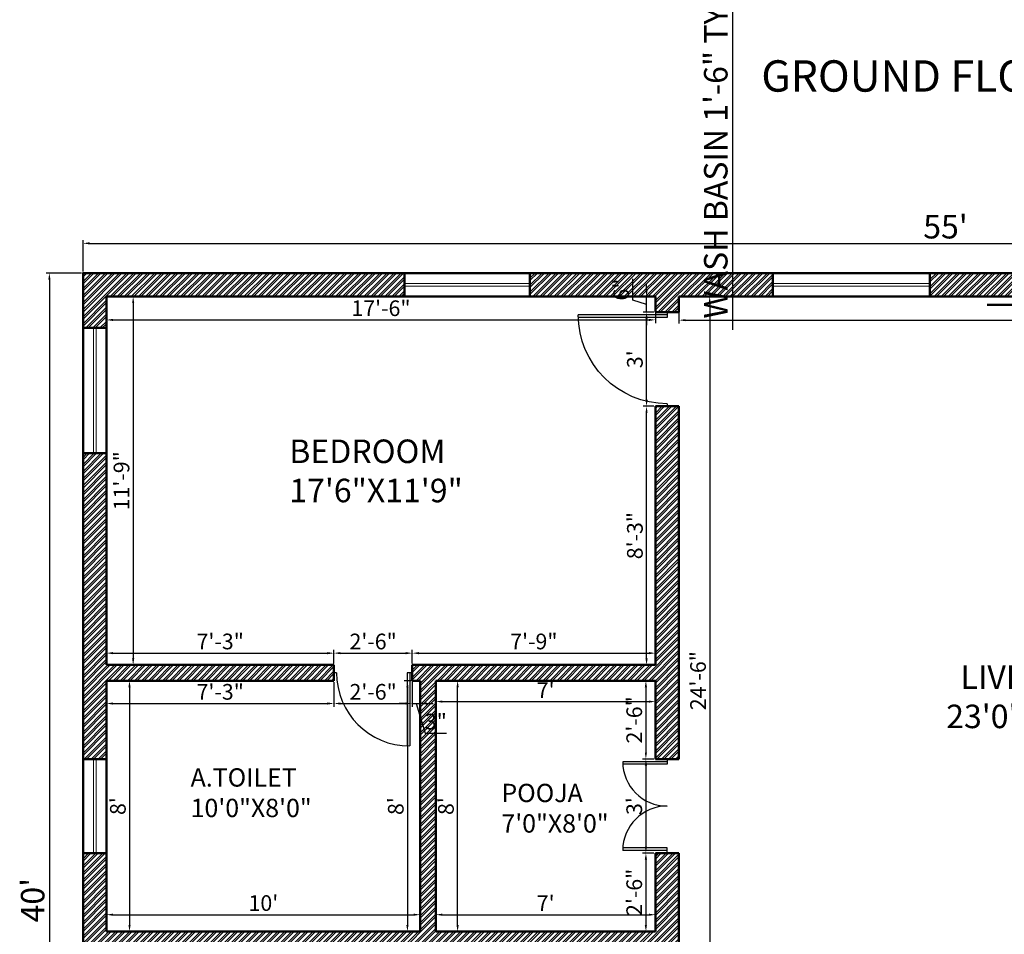
# Model space of a CAD drawing. Units: inches. Extents: x 3590 to 5167, y 65 to 1917.
# Tile 14 of 100: x 3621 to 3998, y 962 to 1312. Entities that reach past the tile are written whole.
import ezdxf

# ---------------------------------------------------------------- set-up
doc = ezdxf.new("R2010")
doc.units = ezdxf.units.IN
for name, color, linetype, lineweight in [('A-ANNO-DIMS', 2, 'Continuous', 18), ('A-ANNO-TEXT', 7, 'Continuous', 25), ('A-AREA-IDEN', 7, 'Continuous', 18), ('A-DOOR', 3, 'Continuous', 25), ('A-GLAZ', 4, 'Continuous', 18), ('A-WALL', 7, 'Continuous', 50), ('A-WALL-PATT', 251, 'Continuous', 13)]:
    doc.layers.add(name, color=color, linetype=linetype, lineweight=lineweight)
doc.styles.get("Standard").update_dxf_attribs({"font": 'arial.ttf'})
doc.dimstyles.new('ISO-25', dxfattribs={"dimtxt": 9, "dimasz": 2.5, "dimexe": 1.25, "dimexo": 0.625, "dimtad": 1, "dimdec": 1, "dimlunit": 3, "dimtxsty": 'Standard', "dimcen": 2.5, "dimadec": 0, "dimazin": 0, "dimtfac": 1, "dimtdec": 1, "dimtmove": 0, "dimatfit": 3, "dimfxl": 1, "dimarcsym": 0})

# ---------------------------------------------------------------- blocks, each defined once
blk = doc.blocks.new('*D9')
at = {"layer": 'A-ANNO-DIMS', "color": 0, "lineweight": -2, "transparency": 16777216}
for p, q in [((3645.51, 1215.97), (3645.51, 1227.96)), ((3648.01, 1226.71), (4303.01, 1226.71)), ((4305.51, 1215.97), (4305.51, 1227.96))]:
    blk.add_line(p, q, dxfattribs=at)
at = {"layer": 'A-ANNO-DIMS', "color": 0, "transparency": 16777216}
for points in [[(3648.01, 1227.13), (3648.01, 1226.29), (3645.51, 1226.71)], [(4303.01, 1227.13), (4303.01, 1226.29), (4305.51, 1226.71)]]:
    blk.add_solid(points, dxfattribs=at)
at = {"layer": 'Defpoints', "color": 0, "transparency": 16777216}
for p in [(4305.51, 1226.71), (3645.51, 1215.35), (4305.51, 1215.35)]:
    blk.add_point(p, dxfattribs=at)
at = {"layer": 'A-ANNO-DIMS', "color": 0, "transparency": 16777216, "insert": (3975.51, 1231.91), "char_height": 9, "attachment_point": 5}
blk.add_mtext("55'", dxfattribs=at)
blk = doc.blocks.new('*D10')
at = {"layer": 'A-ANNO-DIMS', "color": 0, "lineweight": -2, "transparency": 16777216}
for p, q in [((3644.89, 1215.35), (3631.39, 1215.35)), ((3632.64, 1212.85), (3632.64, 737.85)), ((3644.89, 735.35), (3631.39, 735.35))]:
    blk.add_line(p, q, dxfattribs=at)
at = {"layer": 'A-ANNO-DIMS', "color": 0, "transparency": 16777216}
for points in [[(3632.22, 1212.85), (3633.06, 1212.85), (3632.64, 1215.35)], [(3632.22, 737.85), (3633.06, 737.85), (3632.64, 735.35)]]:
    blk.add_solid(points, dxfattribs=at)
at = {"layer": 'Defpoints', "color": 0, "transparency": 16777216}
for p in [(3645.51, 1215.35), (3632.64, 735.35), (3645.51, 735.35)]:
    blk.add_point(p, dxfattribs=at)
at = {"layer": 'A-ANNO-DIMS', "color": 0, "transparency": 16777216, "insert": (3627.42, 975.35), "char_height": 9, "attachment_point": 5, "rotation": 90}
blk.add_mtext("40'", dxfattribs=at)
blk = doc.blocks.new('D1')
for p, q in [((1, 0), (1, 34)), ((2, 0), (2, 33.99)), ((0, 0), (2, 0)), ((35, 0), (36, 0))]:
    blk.add_line(p, q)
at = {"ltscale": 0.5}
blk.add_arc((1, 0), 34, 0, 90, dxfattribs=at)
blk = doc.blocks.new('D2')
for p, q in [((1, 0), (1, 28)), ((2, 0), (2, 27.98)), ((0, 0), (2, 0)), ((29, 0), (30, 0))]:
    blk.add_line(p, q)
at = {"ltscale": 0.5}
blk.add_arc((1, 0), 28, 0, 90, dxfattribs=at)
blk = doc.blocks.new('D3')
for p, q in [((1, 0), (1, 17)), ((2, 0), (2, 16.97)), ((34, 0), (34, 16.97)), ((35, 0), (35, 17)), ((0, 0), (2, 0)), ((36, 0), (34, 0))]:
    blk.add_line(p, q)
at = {"ltscale": 0.5}
for centre, start, end in [((1, 0), 0, 90), ((35, 0), 90, 180)]:
    blk.add_arc(centre, 17, start, end, dxfattribs=at)
blk = doc.blocks.new('*D15')
at = {"layer": 'A-ANNO-DIMS', "color": 0, "lineweight": -2, "transparency": 16777216}
for p, q in [((3654.51, 1205.72), (3654.51, 1196.16)), ((3864.51, 1205.72), (3864.51, 1196.16)), ((3657.01, 1197.41), (3862.01, 1197.41))]:
    blk.add_line(p, q, dxfattribs=at)
at = {"layer": 'A-ANNO-DIMS', "color": 0, "transparency": 16777216}
for points in [[(3657.01, 1197.82), (3657.01, 1196.99), (3654.51, 1197.41)], [(3862.01, 1197.82), (3862.01, 1196.99), (3864.51, 1197.41)]]:
    blk.add_solid(points, dxfattribs=at)
at = {"layer": 'Defpoints', "color": 0, "transparency": 16777216}
for p in [(3654.51, 1206.35), (3864.51, 1206.35), (3864.51, 1197.41)]:
    blk.add_point(p, dxfattribs=at)
at = {"layer": 'A-ANNO-DIMS', "color": 0, "transparency": 16777216, "insert": (3759.51, 1201.1), "char_height": 6, "attachment_point": 5}
blk.add_mtext('17\'-6"', dxfattribs=at)
blk = doc.blocks.new('*D16')
at = {"layer": 'A-ANNO-DIMS', "color": 0, "lineweight": -2, "transparency": 16777216}
for p, q in [((3655.14, 1206.35), (3665.95, 1206.35)), ((3664.7, 1203.85), (3664.7, 1067.85)), ((3655.14, 1065.35), (3665.95, 1065.35))]:
    blk.add_line(p, q, dxfattribs=at)
at = {"layer": 'A-ANNO-DIMS', "color": 0, "transparency": 16777216}
for points in [[(3664.29, 1203.85), (3665.12, 1203.85), (3664.7, 1206.35)], [(3664.29, 1067.85), (3665.12, 1067.85), (3664.7, 1065.35)]]:
    blk.add_solid(points, dxfattribs=at)
at = {"layer": 'Defpoints', "color": 0, "transparency": 16777216}
for p in [(3654.51, 1206.35), (3654.51, 1065.35), (3664.7, 1065.35)]:
    blk.add_point(p, dxfattribs=at)
at = {"layer": 'A-ANNO-DIMS', "color": 0, "transparency": 16777216, "insert": (3661.02, 1135.85), "char_height": 6, "attachment_point": 5, "rotation": 90}
blk.add_mtext('11\'-9"', dxfattribs=at)
blk = doc.blocks.new('*D17')
at = {"layer": 'A-ANNO-DIMS', "color": 0, "lineweight": -2, "transparency": 16777216}
for p, q in [((3654.51, 1065.97), (3654.51, 1071.13)), ((3741.51, 1065.97), (3741.51, 1071.13)), ((3657.01, 1069.88), (3739.01, 1069.88))]:
    blk.add_line(p, q, dxfattribs=at)
at = {"layer": 'A-ANNO-DIMS', "color": 0, "transparency": 16777216}
for points in [[(3657.01, 1070.3), (3657.01, 1069.46), (3654.51, 1069.88)], [(3739.01, 1070.3), (3739.01, 1069.46), (3741.51, 1069.88)]]:
    blk.add_solid(points, dxfattribs=at)
at = {"layer": 'Defpoints', "color": 0, "transparency": 16777216}
for p in [(3741.51, 1069.88), (3654.51, 1065.35), (3741.51, 1065.35)]:
    blk.add_point(p, dxfattribs=at)
at = {"layer": 'A-ANNO-DIMS', "color": 0, "transparency": 16777216, "insert": (3698.01, 1073.57), "char_height": 6, "attachment_point": 5}
blk.add_mtext('7\'-3"', dxfattribs=at)
blk = doc.blocks.new('*D18')
at = {"layer": 'A-ANNO-DIMS', "color": 0, "lineweight": -2, "transparency": 16777216}
for p, q in [((3741.51, 1065.97), (3741.51, 1071.13)), ((3771.51, 1065.97), (3771.51, 1071.13)), ((3744.01, 1069.88), (3769.01, 1069.88))]:
    blk.add_line(p, q, dxfattribs=at)
at = {"layer": 'A-ANNO-DIMS', "color": 0, "transparency": 16777216}
for points in [[(3744.01, 1070.3), (3744.01, 1069.46), (3741.51, 1069.88)], [(3769.01, 1070.3), (3769.01, 1069.46), (3771.51, 1069.88)]]:
    blk.add_solid(points, dxfattribs=at)
at = {"layer": 'Defpoints', "color": 0, "transparency": 16777216}
for p in [(3771.51, 1069.88), (3741.51, 1065.35), (3771.51, 1065.35)]:
    blk.add_point(p, dxfattribs=at)
at = {"layer": 'A-ANNO-DIMS', "color": 0, "transparency": 16777216, "insert": (3756.51, 1073.57), "char_height": 6, "attachment_point": 5}
blk.add_mtext('2\'-6"', dxfattribs=at)
blk = doc.blocks.new('*D19')
at = {"layer": 'A-ANNO-DIMS', "color": 0, "lineweight": -2, "transparency": 16777216}
for p, q in [((3771.51, 1065.97), (3771.51, 1071.13)), ((3864.51, 1065.97), (3864.51, 1071.13)), ((3774.01, 1069.88), (3862.01, 1069.88))]:
    blk.add_line(p, q, dxfattribs=at)
at = {"layer": 'A-ANNO-DIMS', "color": 0, "transparency": 16777216}
for points in [[(3774.01, 1070.3), (3774.01, 1069.46), (3771.51, 1069.88)], [(3862.01, 1070.3), (3862.01, 1069.46), (3864.51, 1069.88)]]:
    blk.add_solid(points, dxfattribs=at)
at = {"layer": 'Defpoints', "color": 0, "transparency": 16777216}
for p in [(3864.51, 1069.88), (3771.51, 1065.35), (3864.51, 1065.35)]:
    blk.add_point(p, dxfattribs=at)
at = {"layer": 'A-ANNO-DIMS', "color": 0, "transparency": 16777216, "insert": (3818.01, 1073.57), "char_height": 6, "attachment_point": 5}
blk.add_mtext('7\'-9"', dxfattribs=at)
blk = doc.blocks.new('*D20')
at = {"layer": 'A-ANNO-DIMS', "color": 0, "lineweight": -2, "transparency": 16777216}
for p, q in [((3863.89, 1164.35), (3859.88, 1164.35)), ((3861.13, 1067.85), (3861.13, 1161.85)), ((3863.89, 1065.35), (3859.88, 1065.35))]:
    blk.add_line(p, q, dxfattribs=at)
at = {"layer": 'A-ANNO-DIMS', "color": 0, "transparency": 16777216}
for points in [[(3860.71, 1161.85), (3861.55, 1161.85), (3861.13, 1164.35)], [(3860.71, 1067.85), (3861.55, 1067.85), (3861.13, 1065.35)]]:
    blk.add_solid(points, dxfattribs=at)
at = {"layer": 'Defpoints', "color": 0, "transparency": 16777216}
for p in [(3861.13, 1164.35), (3864.51, 1164.35), (3864.51, 1065.35)]:
    blk.add_point(p, dxfattribs=at)
at = {"layer": 'A-ANNO-DIMS', "color": 0, "transparency": 16777216, "insert": (3857.44, 1114.85), "char_height": 6, "attachment_point": 5, "rotation": 90}
blk.add_mtext('8\'-3"', dxfattribs=at)
blk = doc.blocks.new('*D21')
at = {"layer": 'A-ANNO-DIMS', "color": 0, "lineweight": -2, "transparency": 16777216}
for p, q in [((3863.89, 1200.35), (3859.88, 1200.35)), ((3861.13, 1166.85), (3861.13, 1197.85)), ((3863.89, 1164.35), (3859.88, 1164.35))]:
    blk.add_line(p, q, dxfattribs=at)
at = {"layer": 'A-ANNO-DIMS', "color": 0, "transparency": 16777216}
for points in [[(3860.71, 1197.85), (3861.55, 1197.85), (3861.13, 1200.35)], [(3860.71, 1166.85), (3861.55, 1166.85), (3861.13, 1164.35)]]:
    blk.add_solid(points, dxfattribs=at)
at = {"layer": 'Defpoints', "color": 0, "transparency": 16777216}
for p in [(3861.13, 1200.35), (3864.51, 1200.35), (3864.51, 1164.35)]:
    blk.add_point(p, dxfattribs=at)
at = {"layer": 'A-ANNO-DIMS', "color": 0, "transparency": 16777216, "insert": (3857.44, 1182.35), "char_height": 6, "attachment_point": 5, "rotation": 90}
blk.add_mtext("3'", dxfattribs=at)
blk = doc.blocks.new('*D22')
at = {"layer": 'A-ANNO-DIMS', "color": 0, "lineweight": -2, "transparency": 16777216}
for p, q in [((3855.88, 1204.92), (3855.88, 1213.1)), ((3861.13, 1208.85), (3861.13, 1211.35)), ((3863.89, 1206.35), (3859.88, 1206.35)), ((3861.13, 1200.35), (3861.13, 1206.35)), ((3861.13, 1200.35), (3861.13, 1206.35)), ((3861.13, 1203.35), (3855.88, 1204.92)), ((3863.89, 1200.35), (3859.88, 1200.35)), ((3861.13, 1197.85), (3861.13, 1195.35))]:
    blk.add_line(p, q, dxfattribs=at)
at = {"layer": 'A-ANNO-DIMS', "color": 0, "transparency": 16777216}
for points in [[(3860.71, 1208.85), (3861.55, 1208.85), (3861.13, 1206.35)], [(3860.71, 1197.85), (3861.55, 1197.85), (3861.13, 1200.35)]]:
    blk.add_solid(points, dxfattribs=at)
at = {"layer": 'Defpoints', "color": 0, "transparency": 16777216}
for p in [(3861.13, 1206.35), (3864.51, 1206.35), (3864.51, 1200.35)]:
    blk.add_point(p, dxfattribs=at)
at = {"layer": 'A-ANNO-DIMS', "color": 0, "transparency": 16777216, "insert": (3852.19, 1209.01), "char_height": 6, "attachment_point": 5, "rotation": 90}
blk.add_mtext('6"', dxfattribs=at)
blk = doc.blocks.new('*D23')
at = {"layer": 'A-ANNO-DIMS', "color": 0, "lineweight": -2, "transparency": 16777216}
for p, q in [((3654.51, 1058.72), (3654.51, 1049.36)), ((3741.51, 1058.72), (3741.51, 1049.36)), ((3657.01, 1050.61), (3739.01, 1050.61))]:
    blk.add_line(p, q, dxfattribs=at)
at = {"layer": 'A-ANNO-DIMS', "color": 0, "transparency": 16777216}
for points in [[(3657.01, 1051.03), (3657.01, 1050.19), (3654.51, 1050.61)], [(3739.01, 1051.03), (3739.01, 1050.19), (3741.51, 1050.61)]]:
    blk.add_solid(points, dxfattribs=at)
at = {"layer": 'Defpoints', "color": 0, "transparency": 16777216}
for p in [(3654.51, 1059.35), (3741.51, 1059.35), (3741.51, 1050.61)]:
    blk.add_point(p, dxfattribs=at)
at = {"layer": 'A-ANNO-DIMS', "color": 0, "transparency": 16777216, "insert": (3698.01, 1054.3), "char_height": 6, "attachment_point": 5}
blk.add_mtext('7\'-3"', dxfattribs=at)
blk = doc.blocks.new('*D24')
at = {"layer": 'A-ANNO-DIMS', "color": 0, "lineweight": -2, "transparency": 16777216}
for p, q in [((3741.51, 1058.72), (3741.51, 1049.36)), ((3771.51, 1058.72), (3771.51, 1049.36)), ((3744.01, 1050.61), (3769.01, 1050.61))]:
    blk.add_line(p, q, dxfattribs=at)
at = {"layer": 'A-ANNO-DIMS', "color": 0, "transparency": 16777216}
for points in [[(3744.01, 1051.03), (3744.01, 1050.19), (3741.51, 1050.61)], [(3769.01, 1051.03), (3769.01, 1050.19), (3771.51, 1050.61)]]:
    blk.add_solid(points, dxfattribs=at)
at = {"layer": 'Defpoints', "color": 0, "transparency": 16777216}
for p in [(3741.51, 1059.35), (3771.51, 1059.35), (3771.51, 1050.61)]:
    blk.add_point(p, dxfattribs=at)
at = {"layer": 'A-ANNO-DIMS', "color": 0, "transparency": 16777216, "insert": (3756.51, 1054.3), "char_height": 6, "attachment_point": 5}
blk.add_mtext('2\'-6"', dxfattribs=at)
blk = doc.blocks.new('*D25')
at = {"layer": 'A-ANNO-DIMS', "color": 0, "lineweight": -2, "transparency": 16777216}
for p, q in [((3771.51, 1058.72), (3771.51, 1049.36)), ((3774.51, 1058.72), (3774.51, 1049.36)), ((3769.01, 1050.61), (3766.51, 1050.61)), ((3771.51, 1050.61), (3774.51, 1050.61)), ((3771.51, 1050.61), (3774.51, 1050.61)), ((3773.01, 1050.61), (3776.43, 1039.23)), ((3777.01, 1050.61), (3779.51, 1050.61)), ((3776.43, 1039.23), (3784.57, 1039.23))]:
    blk.add_line(p, q, dxfattribs=at)
at = {"layer": 'A-ANNO-DIMS', "color": 0, "transparency": 16777216}
for points in [[(3769.01, 1051.03), (3769.01, 1050.19), (3771.51, 1050.61)], [(3777.01, 1051.03), (3777.01, 1050.19), (3774.51, 1050.61)]]:
    blk.add_solid(points, dxfattribs=at)
at = {"layer": 'Defpoints', "color": 0, "transparency": 16777216}
for p in [(3771.51, 1059.35), (3774.51, 1059.35), (3774.51, 1050.61)]:
    blk.add_point(p, dxfattribs=at)
at = {"layer": 'A-ANNO-DIMS', "color": 0, "transparency": 16777216, "insert": (3780.5, 1042.92), "char_height": 6, "attachment_point": 5}
blk.add_mtext('3"', dxfattribs=at)
blk = doc.blocks.new('*D26')
at = {"layer": 'A-ANNO-DIMS', "color": 0, "lineweight": -2, "transparency": 16777216}
for p, q in [((3655.14, 1059.35), (3664.56, 1059.35)), ((3663.31, 1056.85), (3663.31, 965.85)), ((3655.14, 963.35), (3664.56, 963.35))]:
    blk.add_line(p, q, dxfattribs=at)
at = {"layer": 'A-ANNO-DIMS', "color": 0, "transparency": 16777216}
for points in [[(3662.89, 1056.85), (3663.72, 1056.85), (3663.31, 1059.35)], [(3662.89, 965.85), (3663.72, 965.85), (3663.31, 963.35)]]:
    blk.add_solid(points, dxfattribs=at)
at = {"layer": 'Defpoints', "color": 0, "transparency": 16777216}
for p in [(3654.51, 1059.35), (3654.51, 963.35), (3663.31, 963.35)]:
    blk.add_point(p, dxfattribs=at)
at = {"layer": 'A-ANNO-DIMS', "color": 0, "transparency": 16777216, "insert": (3659.62, 1011.35), "char_height": 6, "attachment_point": 5, "rotation": 90}
blk.add_mtext("8'", dxfattribs=at)
blk = doc.blocks.new('*D27')
at = {"layer": 'A-ANNO-DIMS', "color": 0, "lineweight": -2, "transparency": 16777216}
for p, q in [((3654.51, 963.97), (3654.51, 971.04)), ((3657.01, 969.79), (3772.01, 969.79)), ((3774.51, 963.97), (3774.51, 971.04))]:
    blk.add_line(p, q, dxfattribs=at)
at = {"layer": 'A-ANNO-DIMS', "color": 0, "transparency": 16777216}
for points in [[(3657.01, 970.2), (3657.01, 969.37), (3654.51, 969.79)], [(3772.01, 970.2), (3772.01, 969.37), (3774.51, 969.79)]]:
    blk.add_solid(points, dxfattribs=at)
at = {"layer": 'Defpoints', "color": 0, "transparency": 16777216}
for p in [(3774.51, 969.79), (3654.51, 963.35), (3774.51, 963.35)]:
    blk.add_point(p, dxfattribs=at)
at = {"layer": 'A-ANNO-DIMS', "color": 0, "transparency": 16777216, "insert": (3714.51, 973.47), "char_height": 6, "attachment_point": 5}
blk.add_mtext("10'", dxfattribs=at)
blk = doc.blocks.new('*D28')
at = {"layer": 'A-ANNO-DIMS', "color": 0, "lineweight": -2, "transparency": 16777216}
for p, q in [((3780.51, 963.97), (3780.51, 971.04)), ((3783.01, 969.79), (3862.01, 969.79)), ((3864.51, 963.97), (3864.51, 971.04))]:
    blk.add_line(p, q, dxfattribs=at)
at = {"layer": 'A-ANNO-DIMS', "color": 0, "transparency": 16777216}
for points in [[(3783.01, 970.2), (3783.01, 969.37), (3780.51, 969.79)], [(3862.01, 970.2), (3862.01, 969.37), (3864.51, 969.79)]]:
    blk.add_solid(points, dxfattribs=at)
at = {"layer": 'Defpoints', "color": 0, "transparency": 16777216}
for p in [(3864.51, 969.79), (3780.51, 963.35), (3864.51, 963.35)]:
    blk.add_point(p, dxfattribs=at)
at = {"layer": 'A-ANNO-DIMS', "color": 0, "transparency": 16777216, "insert": (3822.51, 973.41), "char_height": 6, "attachment_point": 5}
blk.add_mtext("7'", dxfattribs=at)
blk = doc.blocks.new('*D29')
at = {"layer": 'A-ANNO-DIMS', "color": 0, "lineweight": -2, "transparency": 16777216}
for p, q in [((3781.14, 1059.35), (3790.09, 1059.35)), ((3788.84, 965.85), (3788.84, 1056.85)), ((3781.14, 963.35), (3790.09, 963.35))]:
    blk.add_line(p, q, dxfattribs=at)
at = {"layer": 'A-ANNO-DIMS', "color": 0, "transparency": 16777216}
for points in [[(3788.42, 1056.85), (3789.26, 1056.85), (3788.84, 1059.35)], [(3788.42, 965.85), (3789.26, 965.85), (3788.84, 963.35)]]:
    blk.add_solid(points, dxfattribs=at)
at = {"layer": 'Defpoints', "color": 0, "transparency": 16777216}
for p in [(3780.51, 1059.35), (3788.84, 1059.35), (3780.51, 963.35)]:
    blk.add_point(p, dxfattribs=at)
at = {"layer": 'A-ANNO-DIMS', "color": 0, "transparency": 16777216, "insert": (3785.15, 1011.35), "char_height": 6, "attachment_point": 5, "rotation": 90}
blk.add_mtext("8'", dxfattribs=at)
blk = doc.blocks.new('*D30')
at = {"layer": 'A-ANNO-DIMS', "color": 0, "lineweight": -2, "transparency": 16777216}
for p, q in [((3773.89, 1059.35), (3768.39, 1059.35)), ((3769.64, 1056.85), (3769.64, 965.85)), ((3773.89, 963.35), (3768.39, 963.35))]:
    blk.add_line(p, q, dxfattribs=at)
at = {"layer": 'A-ANNO-DIMS', "color": 0, "transparency": 16777216}
for points in [[(3769.23, 1056.85), (3770.06, 1056.85), (3769.64, 1059.35)], [(3769.23, 965.85), (3770.06, 965.85), (3769.64, 963.35)]]:
    blk.add_solid(points, dxfattribs=at)
at = {"layer": 'Defpoints', "color": 0, "transparency": 16777216}
for p in [(3774.51, 1059.35), (3769.64, 963.35), (3774.51, 963.35)]:
    blk.add_point(p, dxfattribs=at)
at = {"layer": 'A-ANNO-DIMS', "color": 0, "transparency": 16777216, "insert": (3765.96, 1011.35), "char_height": 6, "attachment_point": 5, "rotation": 90}
blk.add_mtext("8'", dxfattribs=at)
blk = doc.blocks.new('*D31')
at = {"layer": 'A-ANNO-DIMS', "color": 0, "lineweight": -2, "transparency": 16777216}
for p, q in [((3780.51, 1058.72), (3780.51, 1050.09)), ((3864.51, 1058.72), (3864.51, 1050.09)), ((3783.01, 1051.34), (3862.01, 1051.34))]:
    blk.add_line(p, q, dxfattribs=at)
at = {"layer": 'A-ANNO-DIMS', "color": 0, "transparency": 16777216}
for points in [[(3783.01, 1051.76), (3783.01, 1050.93), (3780.51, 1051.34)], [(3862.01, 1051.76), (3862.01, 1050.93), (3864.51, 1051.34)]]:
    blk.add_solid(points, dxfattribs=at)
at = {"layer": 'Defpoints', "color": 0, "transparency": 16777216}
for p in [(3780.51, 1059.35), (3864.51, 1059.35), (3864.51, 1051.34)]:
    blk.add_point(p, dxfattribs=at)
at = {"layer": 'A-ANNO-DIMS', "color": 0, "transparency": 16777216, "insert": (3822.51, 1054.97), "char_height": 6, "attachment_point": 5}
blk.add_mtext("7'", dxfattribs=at)
blk = doc.blocks.new('*D32')
at = {"layer": 'A-ANNO-DIMS', "color": 0, "lineweight": -2, "transparency": 16777216}
for p, q in [((3863.89, 1059.35), (3859.63, 1059.35)), ((3860.88, 1056.85), (3860.88, 1031.85)), ((3863.89, 1029.35), (3859.63, 1029.35))]:
    blk.add_line(p, q, dxfattribs=at)
at = {"layer": 'A-ANNO-DIMS', "color": 0, "transparency": 16777216}
for points in [[(3860.46, 1056.85), (3861.29, 1056.85), (3860.88, 1059.35)], [(3860.46, 1031.85), (3861.29, 1031.85), (3860.88, 1029.35)]]:
    blk.add_solid(points, dxfattribs=at)
at = {"layer": 'Defpoints', "color": 0, "transparency": 16777216}
for p in [(3864.51, 1059.35), (3860.88, 1029.35), (3864.51, 1029.35)]:
    blk.add_point(p, dxfattribs=at)
at = {"layer": 'A-ANNO-DIMS', "color": 0, "transparency": 16777216, "insert": (3857.19, 1044.35), "char_height": 6, "attachment_point": 5, "rotation": 90}
blk.add_mtext('2\'-6"', dxfattribs=at)
blk = doc.blocks.new('*D33')
at = {"layer": 'A-ANNO-DIMS', "color": 0, "lineweight": -2, "transparency": 16777216}
for p, q in [((3863.89, 1029.35), (3859.63, 1029.35)), ((3860.88, 1026.85), (3860.88, 995.85)), ((3863.89, 993.35), (3859.63, 993.35))]:
    blk.add_line(p, q, dxfattribs=at)
at = {"layer": 'A-ANNO-DIMS', "color": 0, "transparency": 16777216}
for points in [[(3860.46, 1026.85), (3861.29, 1026.85), (3860.88, 1029.35)], [(3860.46, 995.85), (3861.29, 995.85), (3860.88, 993.35)]]:
    blk.add_solid(points, dxfattribs=at)
at = {"layer": 'Defpoints', "color": 0, "transparency": 16777216}
for p in [(3864.51, 1029.35), (3860.88, 993.35), (3864.51, 993.35)]:
    blk.add_point(p, dxfattribs=at)
at = {"layer": 'A-ANNO-DIMS', "color": 0, "transparency": 16777216, "insert": (3857.19, 1011.35), "char_height": 6, "attachment_point": 5, "rotation": 90}
blk.add_mtext("3'", dxfattribs=at)
blk = doc.blocks.new('*D34')
at = {"layer": 'A-ANNO-DIMS', "color": 0, "lineweight": -2, "transparency": 16777216}
for p, q in [((3863.89, 993.35), (3859.63, 993.35)), ((3860.88, 990.85), (3860.88, 965.85)), ((3863.89, 963.35), (3859.63, 963.35))]:
    blk.add_line(p, q, dxfattribs=at)
at = {"layer": 'A-ANNO-DIMS', "color": 0, "transparency": 16777216}
for points in [[(3860.46, 990.85), (3861.29, 990.85), (3860.88, 993.35)], [(3860.46, 965.85), (3861.29, 965.85), (3860.88, 963.35)]]:
    blk.add_solid(points, dxfattribs=at)
at = {"layer": 'Defpoints', "color": 0, "transparency": 16777216}
for p in [(3864.51, 993.35), (3860.88, 963.35), (3864.51, 963.35)]:
    blk.add_point(p, dxfattribs=at)
at = {"layer": 'A-ANNO-DIMS', "color": 0, "transparency": 16777216, "insert": (3857.19, 978.35), "char_height": 6, "attachment_point": 5, "rotation": 90}
blk.add_mtext('2\'-6"', dxfattribs=at)
blk = doc.blocks.new('*D69')
at = {"layer": 'A-ANNO-DIMS', "color": 0, "lineweight": -2, "transparency": 16777216}
for p, q in [((3873.51, 1205.72), (3873.51, 1196.06)), ((4206.51, 1205.72), (4206.51, 1196.06)), ((3876.01, 1197.31), (4204.01, 1197.31))]:
    blk.add_line(p, q, dxfattribs=at)
at = {"layer": 'A-ANNO-DIMS', "color": 0, "transparency": 16777216}
for points in [[(3876.01, 1197.73), (3876.01, 1196.9), (3873.51, 1197.31)], [(4204.01, 1197.73), (4204.01, 1196.9), (4206.51, 1197.31)]]:
    blk.add_solid(points, dxfattribs=at)
at = {"layer": 'Defpoints', "color": 0, "transparency": 16777216}
for p in [(3873.51, 1206.35), (4206.51, 1206.35), (4206.51, 1197.31)]:
    blk.add_point(p, dxfattribs=at)
at = {"layer": 'A-ANNO-DIMS', "color": 0, "transparency": 16777216, "insert": (4040.01, 1201), "char_height": 6, "attachment_point": 5}
blk.add_mtext('27\'-9"', dxfattribs=at)
blk = doc.blocks.new('*D73')
at = {"layer": 'A-ANNO-DIMS', "color": 0, "lineweight": -2, "transparency": 16777216}
for p, q in [((3874.14, 1206.35), (3886.54, 1206.35)), ((3885.29, 1203.85), (3885.29, 914.85)), ((3874.14, 912.35), (3886.54, 912.35))]:
    blk.add_line(p, q, dxfattribs=at)
at = {"layer": 'A-ANNO-DIMS', "color": 0, "transparency": 16777216}
for points in [[(3884.87, 1203.85), (3885.7, 1203.85), (3885.29, 1206.35)], [(3884.87, 914.85), (3885.7, 914.85), (3885.29, 912.35)]]:
    blk.add_solid(points, dxfattribs=at)
at = {"layer": 'Defpoints', "color": 0, "transparency": 16777216}
for p in [(3873.51, 1206.35), (3873.51, 912.35), (3885.29, 912.35)]:
    blk.add_point(p, dxfattribs=at)
at = {"layer": 'A-ANNO-DIMS', "color": 0, "transparency": 16777216, "insert": (3881.6, 1059.35), "char_height": 6, "attachment_point": 5, "rotation": 90}
blk.add_mtext('24\'-6"', dxfattribs=at)
blk = doc.blocks.new('*D74')
at = {"layer": 'A-ANNO-DIMS', "color": 0, "lineweight": -2, "transparency": 16777216}
for p, q in [((3873.51, 948.97), (3873.51, 959.67)), ((3876.01, 958.42), (4147.01, 958.42)), ((4149.51, 945.97), (4149.51, 959.67))]:
    blk.add_line(p, q, dxfattribs=at)
at = {"layer": 'A-ANNO-DIMS', "color": 0, "transparency": 16777216}
for points in [[(3876.01, 958.83), (3876.01, 958), (3873.51, 958.42)], [(4147.01, 958.83), (4147.01, 958), (4149.51, 958.42)]]:
    blk.add_solid(points, dxfattribs=at)
at = {"layer": 'Defpoints', "color": 0, "transparency": 16777216}
for p in [(4149.51, 958.42), (3873.51, 948.35), (4149.51, 945.35)]:
    blk.add_point(p, dxfattribs=at)
at = {"layer": 'A-ANNO-DIMS', "color": 0, "transparency": 16777216, "insert": (4011.51, 962.11), "char_height": 6, "attachment_point": 5}
blk.add_mtext("23'", dxfattribs=at)
blk = doc.blocks.new('*D306')
at = {"layer": 'A-ANNO-DIMS', "color": 0, "lineweight": -2, "transparency": 16777216}
for p, q in [((3892, 1352.87), (3895.31, 1352.87)), ((3894.06, 1350.37), (3894.06, 1337.5)), ((3892, 1335), (3895.31, 1335)), ((3894.06, 1335), (3894.06, 1193.58))]:
    blk.add_line(p, q, dxfattribs=at)
at = {"layer": 'A-ANNO-DIMS', "color": 0, "transparency": 16777216}
for points in [[(3893.64, 1350.37), (3894.48, 1350.37), (3894.06, 1352.87)], [(3893.64, 1337.5), (3894.48, 1337.5), (3894.06, 1335)]]:
    blk.add_solid(points, dxfattribs=at)
at = {"layer": 'Defpoints', "color": 0, "transparency": 16777216}
for p in [(3891.38, 1352.87), (3891.38, 1335), (3894.06, 1335)]:
    blk.add_point(p, dxfattribs=at)
at = {"layer": 'A-ANNO-DIMS', "color": 0, "transparency": 16777216, "insert": (3888.78, 1263.04), "char_height": 9, "attachment_point": 5, "rotation": 90}
blk.add_mtext('WASH BASIN 1\'-6" TYP.', dxfattribs=at)

msp = doc.modelspace()

# ---------------------------------------------------------------- hatches: boundary and pattern name
at = {"layer": 'A-WALL-PATT', "transparency": 33554687}
h = msp.add_hatch(dxfattribs=at)
h.set_pattern_fill('ANSI32', color=256, scale=0.2)
h.set_pattern_definition([(45, (0, -590.6538), (-1.3470384, 1.3470384), []), (45, (0.898, -590.6538), (-1.3470384, 1.3470384), [])])
h.paths.add_polyline_path([(3768.51, 1215.35), (3645.51, 1215.35), (3645.51, 1194.35), (3654.51, 1194.35), (3654.51, 1206.35), (3671.16, 1206.35), (3768.51, 1206.35)])
h.paths.add_polyline_path([(3909.51, 1215.35), (3816.51, 1215.35), (3816.51, 1206.35), (3864.51, 1206.35), (3864.51, 1200.35), (3873.51, 1200.35), (3873.51, 1206.35), (3909.51, 1206.35)])
h.paths.add_polyline_path([(4053.51, 1215.35), (3969.51, 1215.35), (3969.51, 1206.35), (4053.51, 1206.35)])
h.paths.add_polyline_path([(4215.51, 1215.35), (4113.51, 1215.35), (4113.51, 1206.35), (4206.51, 1206.35), (4206.51, 1200.35), (4215.51, 1200.35)])
h.paths.add_polyline_path([(3654.51, 1146.35), (3645.51, 1146.35), (3645.51, 1029.35), (3654.51, 1029.35), (3654.51, 1059.35), (3741.51, 1059.35), (3741.51, 1065.35), (3654.51, 1065.35)], flags=17)
h.paths.add_polyline_path([(3873.51, 1164.35), (3864.51, 1164.35), (3864.51, 1065.35), (3771.51, 1065.35), (3771.51, 1059.35), (3774.51, 1059.35), (3774.51, 963.35), (3654.51, 963.35), (3654.51, 993.35), (3645.51, 993.35), (3645.51, 948.35), (3654.51, 948.35), (3654.51, 954.35), (3864.51, 954.35), (3864.51, 948.35), (3873.51, 948.35), (3873.51, 993.35), (3864.51, 993.35), (3864.51, 963.35), (3780.51, 963.35), (3780.51, 1059.35), (3864.51, 1059.35), (3864.51, 1029.35), (3873.51, 1029.35)])
h.paths.add_polyline_path([(3654.51, 900.35), (3645.51, 900.35), (3645.51, 735.35), (3810.51, 735.35), (3810.51, 744.35), (3809.96, 744.35), (3654.51, 744.35)])
h.paths.add_polyline_path([(3915.51, 744.35), (3873.51, 744.35), (3873.51, 762.21), (3873.51, 831.35), (3876.51, 831.35), (3876.51, 840.35), (3864.51, 840.35), (3864.51, 744.35), (3858.51, 744.35), (3858.51, 735.35), (3915.51, 735.35)])
h.paths.add_polyline_path([(4028.01, 744.35), (4002.51, 744.35), (4002.51, 912.35), (3981.51, 912.35), (3981.51, 903.35), (3993.51, 903.35), (3993.51, 840.35), (3921.51, 840.35), (3921.51, 903.35), (3933.51, 903.35), (3933.51, 912.35), (3864.51, 912.35), (3864.51, 903.35), (3912.51, 903.35), (3912.51, 840.35), (3906.51, 840.35), (3906.51, 831.35), (3993.51, 831.35), (3993.51, 744.35), (3951.51, 744.35), (3951.51, 735.35), (4028.01, 735.35)])
h.paths.add_polyline_path([(4203.51, 744.35), (4158.51, 744.35), (4158.51, 936.35), (4194.51, 936.35), (4194.51, 945.35), (4149.51, 945.35), (4149.51, 744.35), (4124.01, 744.35), (4124.01, 735.35), (4203.51, 735.35)])
h.paths.add_polyline_path([(4305.51, 975.35), (4296.51, 975.35), (4296.51, 945.35), (4278.64, 945.35), (4260.51, 945.35), (4260.51, 936.35), (4296.51, 936.35), (4296.51, 930.35), (4305.51, 930.35)])
h.paths.add_polyline_path([(4305.51, 882.35), (4296.51, 882.35), (4296.51, 744.35), (4251.51, 744.35), (4251.51, 735.35), (4305.51, 735.35)])
h.paths.add_polyline_path([(4305.51, 1086.35), (4215.51, 1086.35), (4215.51, 1152.35), (4206.51, 1152.35), (4206.51, 1086.35), (4149.51, 1086.35), (4149.51, 1077.35), (4296.51, 1077.35), (4296.51, 1047.35), (4305.51, 1047.35)])

# ---------------------------------------------------------------- linework, layer by layer
at = {"layer": 'A-GLAZ'}
for p, q in [((3816.51, 1211.35), (3768.51, 1211.35)), ((3816.51, 1210.35), (3768.51, 1210.35)), ((3969.51, 1211.35), (3909.51, 1211.35)), ((3969.51, 1210.35), (3909.51, 1210.35)), ((3649.51, 1146.35), (3649.51, 1194.35)), ((3650.51, 1146.35), (3650.51, 1194.35)), ((3649.51, 993.35), (3649.51, 1029.35)), ((3650.51, 993.35), (3650.51, 1029.35))]:
    msp.add_line(p, q, dxfattribs=at)
at = {"layer": 'A-WALL'}
for p, q in [((3768.51, 1206.35), (3768.51, 1215.35)), ((3816.51, 1206.35), (3816.51, 1215.35)), ((3909.51, 1206.35), (3909.51, 1215.35)), ((3969.51, 1206.35), (3969.51, 1215.35)), ((3654.51, 1206.35), (3864.51, 1206.35)), ((3654.51, 1065.35), (3654.51, 1206.35)), ((3864.51, 1200.35), (3864.51, 1206.35)), ((3873.51, 1206.35), (4206.51, 1206.35)), ((3873.51, 1200.35), (3873.51, 1206.35)), ((3991.51, 1203.16), (4031.51, 1203.16)), ((3864.51, 1200.35), (3873.51, 1200.35)), ((3654.51, 1194.35), (3645.51, 1194.35)), ((3864.51, 1164.35), (3873.51, 1164.35)), ((3864.51, 1065.35), (3864.51, 1164.35)), ((3873.51, 1029.35), (3873.51, 1164.35)), ((3654.51, 1146.35), (3645.51, 1146.35)), ((3654.51, 1065.35), (3741.51, 1065.35)), ((3741.51, 1059.35), (3741.51, 1065.35)), ((3771.51, 1065.35), (3864.51, 1065.35)), ((3771.51, 1059.35), (3771.51, 1065.35)), ((3654.51, 1059.35), (3741.51, 1059.35)), ((3654.51, 963.35), (3654.51, 1059.35)), ((3771.51, 1059.35), (3774.51, 1059.35)), ((3774.51, 963.35), (3774.51, 1059.35)), ((3780.51, 1059.35), (3864.51, 1059.35)), ((3780.51, 963.35), (3780.51, 1059.35)), ((3864.51, 1029.35), (3864.51, 1059.35)), ((3654.51, 1029.35), (3645.51, 1029.35)), ((3864.51, 1029.35), (3873.51, 1029.35)), ((3654.51, 993.35), (3645.51, 993.35)), ((3864.51, 963.35), (3864.51, 993.35)), ((3864.51, 993.35), (3873.51, 993.35)), ((3873.51, 948.35), (3873.51, 993.35)), ((3774.51, 963.35), (3654.51, 963.35)), ((3864.51, 963.35), (3780.51, 963.35))]:
    msp.add_line(p, q, dxfattribs=at)
msp.add_lwpolyline([(4305.51, 1086.35), (4305.51, 735.35), (3645.51, 735.35), (3645.51, 1215.35), (4215.51, 1215.35)], dxfattribs=at)

# ---------------------------------------------------------------- block references
at = {"layer": 'A-DOOR', "xscale": -1, "rotation": 90}
msp.add_blockref('D1', (3869.01, 1200.35), dxfattribs=at)
at = {"layer": 'A-DOOR'}
for name, p, rotation in [('D2', (3771.51, 1062.35), 180), ('D3', (3869.01, 993.35), 90)]:
    msp.add_blockref(name, p, dxfattribs=dict(at, rotation=rotation))

# ---------------------------------------------------------------- texts
at = {"layer": 'A-ANNO-TEXT', "insert": (3905.03, 1296.76), "char_height": 12, "attachment_point": 1}
msp.add_mtext_dynamic_manual_height_columns('{\\fTimes New Roman|b0|i0|c0|p18;GROUND FLOOR PLAN}', width=197.6934, gutter_width=12.5, heights=[0], dxfattribs=at)
at = {"layer": 'A-AREA-IDEN', "attachment_point": 1}
for s, insert, char_height in [('{\\fTimes New Roman|b0|i0|c0|p18;BEDROOM\\P17\'6"X11\'9"}', (3724.44, 1151.63), 9), ('{\\fTimes New Roman|b0|i0|c0|p18;  LIVING\\P23\'0"X24\'6"}', (3975.77, 1065.18), 9), ('{\\fTimes New Roman|b0|i0|c0|p18;A.TOILET\\P10\'0"X8\'0"}', (3686.68, 1025.81), 7), ('{\\fTimes New Roman|b0|i0|c0|p18;POOJA\\P7\'0"X8\'0"}', (3805.59, 1019.88), 7)]:
    msp.add_mtext_dynamic_manual_height_columns(s, width=67.3508, gutter_width=12.5, heights=[0], dxfattribs=dict(at, insert=insert, char_height=char_height))

# ---------------------------------------------------------------- dimensions: what is measured, and where the dimension line sits
at = {"layer": 'A-ANNO-DIMS'}
dim = msp.add_linear_dim(base=(3894.06, 1335), p1=(3891.38, 1352.87), p2=(3891.38, 1335), angle=270, text='WASH BASIN <> TYP.', dimstyle='ISO-25', override={"dimdec": 1, "dimlfac": 1, "dimrnd": 0, "dimzin": 1, "dimdsep": 46, "dimlunit": 4, "dimfrac": 2}, dxfattribs=at)
dim.commit()
dim.dimension.update_dxf_attribs({"geometry": '*D306', "text_midpoint": (3888.78, 1263.04)})
for base, p1, p2, override, picture, middle in [((4305.51, 1226.71), (3645.51, 1215.35), (4305.51, 1215.35), {"dimclrd": 0, "dimclre": 0, "dimclrt": 0}, '*D9', (3975.51, 1231.91)), ((3864.51, 1197.41), (3654.51, 1206.35), (3864.51, 1206.35), {"dimtxt": 6, "dimclrd": 0, "dimclre": 0, "dimclrt": 0}, '*D15', (3759.51, 1201.1)), ((4206.51, 1197.31), (3873.51, 1206.35), (4206.51, 1206.35), {"dimtxt": 6, "dimclrd": 0, "dimclre": 0, "dimclrt": 0}, '*D69', (4040.01, 1201)), ((3741.51, 1069.88), (3654.51, 1065.35), (3741.51, 1065.35), {"dimtxt": 6, "dimclrd": 0, "dimclre": 0, "dimclrt": 0}, '*D17', (3698.01, 1073.57)), ((3771.51, 1069.88), (3741.51, 1065.35), (3771.51, 1065.35), {"dimtxt": 6, "dimclrd": 0, "dimclre": 0, "dimclrt": 0, "dimtmove": 1}, '*D18', (3756.51, 1073.57)), ((3864.51, 1069.88), (3771.51, 1065.35), (3864.51, 1065.35), {"dimtxt": 6, "dimclrd": 0, "dimclre": 0, "dimclrt": 0, "dimtmove": 1}, '*D19', (3818.01, 1073.57)), ((3741.51, 1050.61), (3654.51, 1059.35), (3741.51, 1059.35), {"dimtxt": 6, "dimclrd": 0, "dimclre": 0, "dimclrt": 0}, '*D23', (3698.01, 1054.3)), ((3771.51, 1050.61), (3741.51, 1059.35), (3771.51, 1059.35), {"dimtxt": 6, "dimclrd": 0, "dimclre": 0, "dimclrt": 0, "dimtmove": 1}, '*D24', (3756.51, 1054.3)), ((3774.51, 1050.61), (3771.51, 1059.35), (3774.51, 1059.35), {"dimtxt": 6, "dimclrd": 0, "dimclre": 0, "dimclrt": 0, "dimtmove": 1}, '*D25', (3777.05, 1042.92)), ((3864.51, 1051.34), (3780.51, 1059.35), (3864.51, 1059.35), {"dimtxt": 6, "dimclrd": 0, "dimclre": 0, "dimclrt": 0}, '*D31', (3822.51, 1054.97)), ((3774.51, 969.79), (3654.51, 963.35), (3774.51, 963.35), {"dimtxt": 6, "dimclrd": 0, "dimclre": 0, "dimclrt": 0}, '*D27', (3714.51, 973.47)), ((3864.51, 969.79), (3780.51, 963.35), (3864.51, 963.35), {"dimtxt": 6, "dimclrd": 0, "dimclre": 0, "dimclrt": 0}, '*D28', (3822.51, 973.41)), ((4149.51, 958.42), (3873.51, 948.35), (4149.51, 945.35), {"dimtxt": 6, "dimclrd": 0, "dimclre": 0, "dimclrt": 0}, '*D74', (4011.51, 962.11))]:
    dim = msp.add_linear_dim(base=base, p1=p1, p2=p2, dimstyle='ISO-25', override=override, dxfattribs=at)
    dim.commit()
    dim.dimension.update_dxf_attribs({"geometry": picture, "text_midpoint": middle})
for base, p1, p2, override, picture, middle in [((3632.64, 735.35), (3645.51, 1215.35), (3645.51, 735.35), {"dimclrd": 0, "dimclre": 0, "dimclrt": 0}, '*D10', (3627.42, 975.35)), ((3861.13, 1206.35), (3864.51, 1200.35), (3864.51, 1206.35), {"dimtxt": 6, "dimclrd": 0, "dimclre": 0, "dimclrt": 0, "dimtmove": 1}, '*D22', (3852.19, 1205.55)), ((3664.7, 1065.35), (3654.51, 1206.35), (3654.51, 1065.35), {"dimtxt": 6, "dimclrd": 0, "dimclre": 0, "dimclrt": 0}, '*D16', (3661.02, 1135.85)), ((3885.29, 912.35), (3873.51, 1206.35), (3873.51, 912.35), {"dimtxt": 6, "dimclrd": 0, "dimclre": 0, "dimclrt": 0}, '*D73', (3881.6, 1059.35)), ((3861.13, 1200.35), (3864.51, 1164.35), (3864.51, 1200.35), {"dimtxt": 6, "dimclrd": 0, "dimclre": 0, "dimclrt": 0, "dimtmove": 1}, '*D21', (3857.44, 1182.35)), ((3861.13, 1164.35), (3864.51, 1065.35), (3864.51, 1164.35), {"dimtxt": 6, "dimclrd": 0, "dimclre": 0, "dimclrt": 0}, '*D20', (3857.44, 1114.85)), ((3663.31, 963.35), (3654.51, 1059.35), (3654.51, 963.35), {"dimtxt": 6, "dimclrd": 0, "dimclre": 0, "dimclrt": 0}, '*D26', (3659.62, 1011.35)), ((3769.64, 963.35), (3774.51, 1059.35), (3774.51, 963.35), {"dimtxt": 6, "dimclrd": 0, "dimclre": 0, "dimclrt": 0}, '*D30', (3765.96, 1011.35)), ((3788.84, 1059.35), (3780.51, 963.35), (3780.51, 1059.35), {"dimtxt": 6, "dimclrd": 0, "dimclre": 0, "dimclrt": 0}, '*D29', (3785.15, 1011.35)), ((3860.88, 1029.35), (3864.51, 1059.35), (3864.51, 1029.35), {"dimtxt": 6, "dimclrd": 0, "dimclre": 0, "dimclrt": 0}, '*D32', (3857.19, 1044.35)), ((3860.88, 993.35), (3864.51, 1029.35), (3864.51, 993.35), {"dimtxt": 6, "dimclrd": 0, "dimclre": 0, "dimclrt": 0, "dimtmove": 1}, '*D33', (3857.19, 1011.35)), ((3860.88, 963.35), (3864.51, 993.35), (3864.51, 963.35), {"dimtxt": 6, "dimclrd": 0, "dimclre": 0, "dimclrt": 0, "dimtmove": 1}, '*D34', (3857.19, 978.35))]:
    dim = msp.add_linear_dim(base=base, p1=p1, p2=p2, angle=90, dimstyle='ISO-25', override=override, dxfattribs=at)
    dim.commit()
    dim.dimension.update_dxf_attribs({"geometry": picture, "text_midpoint": middle})

doc.saveas('drawing.dxf')
